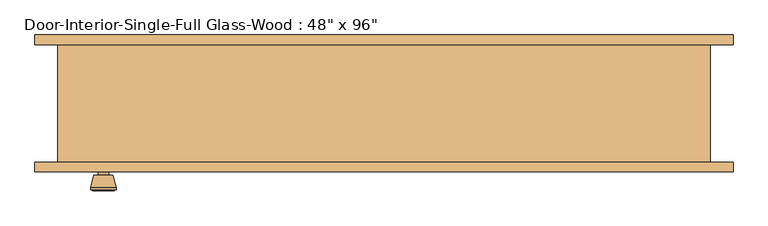
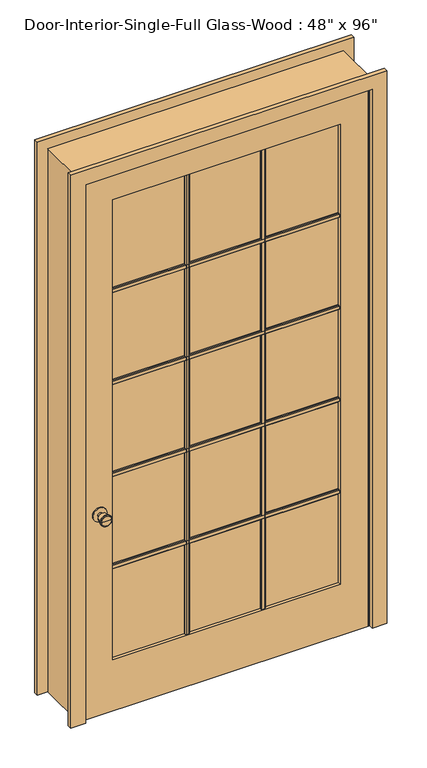
"""IFC4 building model written with IfcOpenShell, lengths in millimetres: door geometry."""

from ifc_helpers import new_model, si_unit, point, frame, frame_2d, origin, place, context, project, spatial, polyline, circle_curve, trimmed, segment, composite_curve, outline, extrude, faceted_brep, source, transform, mapped, element, save
from ifc_brep_helpers import plane_surface, cylinder_surface, revolved_surface, advanced_brep


def door_6ee39103(model_context):
    return source(origin(), model_context, "Body", "SolidModel", [
        extrude(outline(polyline([(-97.155, 1911.35), (-97.155, 1892.3), (-103.505, 1892.3), (-106.68, 1895.475), (-106.68, 1908.175), (-103.505, 1911.35), (-97.155, 1911.35)])), frame((-488.95, 0.0, 0.0), z_axis=(1.0, 0.0, 0.0), x_axis=(0.0, 1.0, 0.0)), (0.0, 0.0, 1.0), 977.9),
        extrude(outline(polyline([(-97.155, 1493.8375), (-97.155, 1474.7875), (-103.505, 1474.7875), (-106.68, 1477.9625), (-106.68, 1490.6625), (-103.505, 1493.8375), (-97.155, 1493.8375)])), frame((-488.95, 0.0, 0.0), z_axis=(1.0, 0.0, 0.0), x_axis=(0.0, 1.0, 0.0)), (0.0, 0.0, 1.0), 977.9),
        extrude(outline(polyline([(-97.155, 1076.325), (-97.155, 1057.275), (-103.505, 1057.275), (-106.68, 1060.45), (-106.68, 1073.15), (-103.505, 1076.325), (-97.155, 1076.325)])), frame((-488.95, 0.0, 0.0), z_axis=(1.0, 0.0, 0.0), x_axis=(0.0, 1.0, 0.0)), (0.0, 0.0, 1.0), 977.9),
        extrude(outline(polyline([(-97.155, 658.8125), (-97.155, 639.7625), (-103.505, 639.7625), (-106.68, 642.9375), (-106.68, 655.6375), (-103.505, 658.8125), (-97.155, 658.8125)])), frame((-488.95, 0.0, 0.0), z_axis=(1.0, 0.0, 0.0), x_axis=(0.0, 1.0, 0.0)), (0.0, 0.0, 1.0), 977.9),
        extrude(outline(polyline([(153.4583333, -97.155), (172.5083333, -97.155), (172.5083333, -103.505), (169.3333333, -106.68), (156.6333333, -106.68), (153.4583333, -103.505), (153.4583333, -97.155)])), frame((0.0, 0.0, 231.775), z_axis=(0.0, 0.0, 1.0), x_axis=(1.0, 0.0, 0.0)), (0.0, 0.0, 1.0), 2087.5625),
        extrude(outline(polyline([(-172.5083333, -97.155), (-153.4583333, -97.155), (-153.4583333, -103.505), (-156.6333333, -106.68), (-169.3333333, -106.68), (-172.5083333, -103.505), (-172.5083333, -97.155)])), frame((0.0, 0.0, 231.775), z_axis=(0.0, 0.0, 1.0), x_axis=(1.0, 0.0, 0.0)), (0.0, 0.0, 1.0), 2087.5625),
        extrude(outline(polyline([(-90.17, 1911.35), (-83.82, 1911.35), (-80.645, 1908.175), (-80.645, 1895.475), (-83.82, 1892.3), (-90.17, 1892.3), (-90.17, 1911.35)])), frame((-488.95, 0.0, 0.0), z_axis=(1.0, 0.0, 0.0), x_axis=(0.0, 1.0, 0.0)), (0.0, 0.0, 1.0), 977.9),
        extrude(outline(polyline([(-90.17, 1493.8375), (-83.82, 1493.8375), (-80.645, 1490.6625), (-80.645, 1477.9625), (-83.82, 1474.7875), (-90.17, 1474.7875), (-90.17, 1493.8375)])), frame((-488.95, 0.0, 0.0), z_axis=(1.0, 0.0, 0.0), x_axis=(0.0, 1.0, 0.0)), (0.0, 0.0, 1.0), 977.9),
        extrude(outline(polyline([(-90.17, 1076.325), (-83.82, 1076.325), (-80.645, 1073.15), (-80.645, 1060.45), (-83.82, 1057.275), (-90.17, 1057.275), (-90.17, 1076.325)])), frame((-488.95, 0.0, 0.0), z_axis=(1.0, 0.0, 0.0), x_axis=(0.0, 1.0, 0.0)), (0.0, 0.0, 1.0), 977.9),
        extrude(outline(polyline([(-90.17, 658.8125), (-83.82, 658.8125), (-80.645, 655.6375), (-80.645, 642.9375), (-83.82, 639.7625), (-90.17, 639.7625), (-90.17, 658.8125)])), frame((-488.95, 0.0, 0.0), z_axis=(1.0, 0.0, 0.0), x_axis=(0.0, 1.0, 0.0)), (0.0, 0.0, 1.0), 977.9),
        extrude(outline(polyline([(153.4583333, -90.17), (153.4583333, -83.82), (156.6333333, -80.645), (169.3333333, -80.645), (172.5083333, -83.82), (172.5083333, -90.17), (153.4583333, -90.17)])), frame((0.0, 0.0, 231.775), z_axis=(0.0, 0.0, 1.0), x_axis=(1.0, 0.0, 0.0)), (0.0, 0.0, 1.0), 2087.5625),
        extrude(outline(polyline([(-172.5083333, -90.17), (-172.5083333, -83.82), (-169.3333333, -80.645), (-156.6333333, -80.645), (-153.4583333, -83.82), (-153.4583333, -90.17), (-172.5083333, -90.17)])), frame((0.0, 0.0, 231.775), z_axis=(0.0, 0.0, 1.0), x_axis=(1.0, 0.0, 0.0)), (0.0, 0.0, 1.0), 2087.5625),
        advanced_brep(
        [(-546.1, -70.2, 914.4), (-556.1, -70.2, 914.4), (-536.1, -70.2, 914.4), (-525.6241324, -21.2, 914.4), (-566.5758676, -21.2, 914.4), (-546.1, -21.2, 914.4), (-521.1, -23.0278681, 914.4), (-571.1, -23.0278681, 914.4), (-521.1, -26.4915463, 914.4), (-571.1, -26.4915463, 914.4), (-527.463764, -51.2, 914.4), (-564.736236, -51.2, 914.4), (-536.1, -51.2, 914.4), (-556.1, -51.2, 914.4)],
        [
            (0, 1),
            (1, 2, circle_curve(frame((-546.1, -70.2, 914.4), z_axis=(0.0, -1.0, 0.0), x_axis=(-1.0, 0.0, 0.0)), 10.0)),
            (2, 0),
            (2, 1, circle_curve(frame((-546.1, -70.2, 914.4), z_axis=(0.0, -1.0, 0.0), x_axis=(-1.0, 0.0, 0.0)), 10.0)),
            (3, 4, circle_curve(frame((-546.1, -21.2, 914.4), z_axis=(0.0, 1.0, 0.0), x_axis=(-1.0, 0.0, 0.0)), 20.4758676)),
            (4, 5),
            (5, 3),
            (4, 3, circle_curve(frame((-546.1, -21.2, 914.4), z_axis=(0.0, 1.0, 0.0), x_axis=(-1.0, 0.0, 0.0)), 20.4758676)),
            (6, 7, circle_curve(frame((-546.1, -23.0278681, 914.4), z_axis=(0.0, 1.0, 0.0), x_axis=(-1.0, 0.0, 0.0)), 25.0)),
            (7, 4),
            (3, 6),
            (7, 6, circle_curve(frame((-546.1, -23.0278681, 914.4), z_axis=(0.0, 1.0, 0.0), x_axis=(-1.0, 0.0, 0.0)), 25.0)),
            (8, 9, circle_curve(frame((-546.1, -26.4915463, 914.4), z_axis=(0.0, 1.0, 0.0), x_axis=(-1.0, 0.0, 0.0)), 25.0)),
            (9, 7),
            (6, 8),
            (9, 8, circle_curve(frame((-546.1, -26.4915463, 914.4), z_axis=(0.0, 1.0, 0.0), x_axis=(-1.0, 0.0, 0.0)), 25.0)),
            (10, 11, circle_curve(frame((-546.1, -51.2, 914.4), z_axis=(0.0, 1.0, 0.0), x_axis=(-1.0, 0.0, 0.0)), 18.636236)),
            (11, 9),
            (8, 10),
            (11, 10, circle_curve(frame((-546.1, -51.2, 914.4), z_axis=(0.0, 1.0, 0.0), x_axis=(-1.0, 0.0, 0.0)), 18.636236)),
            (12, 13, circle_curve(frame((-546.1, -51.2, 914.4), z_axis=(0.0, 1.0, 0.0), x_axis=(-1.0, 0.0, 0.0)), 10.0)),
            (13, 11),
            (10, 12),
            (13, 12, circle_curve(frame((-546.1, -51.2, 914.4), z_axis=(0.0, 1.0, 0.0), x_axis=(-1.0, 0.0, 0.0)), 10.0)),
            (1, 13),
            (12, 2),
        ],
        [
            plane_surface(frame((-546.1, -70.2, 914.4), z_axis=(0.0, -1.0, 0.0), x_axis=(-1.0, 0.0, 0.0))),
            plane_surface(frame((-546.1, -21.2, 914.4), z_axis=(0.0, 1.0, 0.0), x_axis=(-1.0, 0.0, 0.0))),
            revolved_surface(polyline([(-566.5758676, -21.2, 914.4), (-571.1, -23.0278681, 914.4)]), (-546.1, -70.2, 914.4), (0.0, -1.0, 0.0)),
            cylinder_surface(frame((-546.1, -70.2, 914.4), z_axis=(0.0, -1.0, 0.0), x_axis=(-1.0, 0.0, 0.0)), 25.0),
            revolved_surface(polyline([(-571.1, -26.4915463, 914.4), (-564.736236, -51.2, 914.4)]), (-546.1, -70.2, 914.4), (0.0, -1.0, 0.0)),
            plane_surface(frame((-546.1, -51.2, 914.4), z_axis=(0.0, -1.0, 0.0), x_axis=(-1.0, 0.0, 0.0))),
            cylinder_surface(frame((-546.1, -70.2, 914.4), z_axis=(0.0, -1.0, 0.0), x_axis=(-1.0, 0.0, 0.0)), 10.0),
        ],
        [
            (0, [[1, 2, 3]]),
            (0, [[-3, 4, -1]]),
            (1, [[5, 6, 7]]),
            (1, [[8, -7, -6]]),
            (2, [[9, 10, -5, 11]]),
            (2, [[12, -11, -8, -10]]),
            (3, [[13, 14, -9, 15]]),
            (3, [[16, -15, -12, -14]]),
            (4, [[17, 18, -13, 19]]),
            (4, [[20, -19, -16, -18]]),
            (5, [[21, 22, -17, 23]]),
            (5, [[24, -23, -20, -22]]),
            (6, [[-2, 25, -21, 26]]),
            (6, [[-4, -26, -24, -25]]),
        ],
    ),
        extrude(outline(composite_curve([segment(trimmed(circle_curve(frame_2d((914.4, -546.1)), 30.0), [point((914.4, -576.1))], [point((914.4, -516.1))], False, "CARTESIAN"), True, "CONTINUOUS"), segment(trimmed(circle_curve(frame_2d((914.4, -546.1)), 30.0), [point((914.4, -516.1))], [point((914.4, -576.1))], False, "CARTESIAN"), True, "CONTINUOUS")], self_intersect=False)), frame((0.0, -76.2, 0.0), z_axis=(0.0, 1.0, 0.0), x_axis=(0.0, 0.0, 1.0)), (0.0, 0.0, 1.0), 6.0),
        advanced_brep(
        [(-546.1, -117.125, 914.4), (-536.1, -117.125, 914.4), (-556.1, -117.125, 914.4), (-525.6241324, -166.125, 914.4), (-546.1, -166.125, 914.4), (-566.5758676, -166.125, 914.4), (-521.1, -164.2971319, 914.4), (-571.1, -164.2971319, 914.4), (-521.1, -160.8334537, 914.4), (-571.1, -160.8334537, 914.4), (-527.463764, -136.125, 914.4), (-564.736236, -136.125, 914.4), (-536.1, -136.125, 914.4), (-556.1, -136.125, 914.4)],
        [
            (0, 1),
            (1, 2, circle_curve(frame((-546.1, -117.125, 914.4), z_axis=(0.0, 1.0, 0.0), x_axis=(-1.0, 0.0, 0.0)), 10.0)),
            (2, 0),
            (2, 1, circle_curve(frame((-546.1, -117.125, 914.4), z_axis=(0.0, 1.0, 0.0), x_axis=(-1.0, 0.0, 0.0)), 10.0)),
            (3, 4),
            (4, 5),
            (5, 3, circle_curve(frame((-546.1, -166.125, 914.4), z_axis=(0.0, -1.0, 0.0), x_axis=(-1.0, 0.0, 0.0)), 20.4758676)),
            (3, 5, circle_curve(frame((-546.1, -166.125, 914.4), z_axis=(0.0, -1.0, 0.0), x_axis=(-1.0, 0.0, 0.0)), 20.4758676)),
            (6, 3),
            (5, 7),
            (7, 6, circle_curve(frame((-546.1, -164.2971319, 914.4), z_axis=(0.0, -1.0, 0.0), x_axis=(-1.0, 0.0, 0.0)), 25.0)),
            (6, 7, circle_curve(frame((-546.1, -164.2971319, 914.4), z_axis=(0.0, -1.0, 0.0), x_axis=(-1.0, 0.0, 0.0)), 25.0)),
            (8, 6),
            (7, 9),
            (9, 8, circle_curve(frame((-546.1, -160.8334537, 914.4), z_axis=(0.0, -1.0, 0.0), x_axis=(-1.0, 0.0, 0.0)), 25.0)),
            (8, 9, circle_curve(frame((-546.1, -160.8334537, 914.4), z_axis=(0.0, -1.0, 0.0), x_axis=(-1.0, 0.0, 0.0)), 25.0)),
            (10, 8),
            (9, 11),
            (11, 10, circle_curve(frame((-546.1, -136.125, 914.4), z_axis=(0.0, -1.0, 0.0), x_axis=(-1.0, 0.0, 0.0)), 18.636236)),
            (10, 11, circle_curve(frame((-546.1, -136.125, 914.4), z_axis=(0.0, -1.0, 0.0), x_axis=(-1.0, 0.0, 0.0)), 18.636236)),
            (12, 10),
            (11, 13),
            (13, 12, circle_curve(frame((-546.1, -136.125, 914.4), z_axis=(0.0, -1.0, 0.0), x_axis=(-1.0, 0.0, 0.0)), 10.0)),
            (12, 13, circle_curve(frame((-546.1, -136.125, 914.4), z_axis=(0.0, -1.0, 0.0), x_axis=(-1.0, 0.0, 0.0)), 10.0)),
            (1, 12),
            (13, 2),
        ],
        [
            plane_surface(frame((-546.1, -117.125, 914.4), z_axis=(0.0, 1.0, 0.0), x_axis=(-1.0, 0.0, 0.0))),
            plane_surface(frame((-546.1, -166.125, 914.4), z_axis=(0.0, -1.0, 0.0), x_axis=(-1.0, 0.0, 0.0))),
            revolved_surface(polyline([(-566.5758676, -166.125, 914.4), (-571.1, -164.2971319, 914.4)]), (-546.1, -117.125, 914.4), (0.0, 1.0, 0.0)),
            cylinder_surface(frame((-546.1, -117.125, 914.4), z_axis=(0.0, 1.0, 0.0), x_axis=(-1.0, 0.0, 0.0)), 25.0),
            revolved_surface(polyline([(-571.1, -160.8334537, 914.4), (-564.736236, -136.125, 914.4)]), (-546.1, -117.125, 914.4), (0.0, 1.0, 0.0)),
            plane_surface(frame((-546.1, -136.125, 914.4), z_axis=(0.0, 1.0, 0.0), x_axis=(-1.0, 0.0, 0.0))),
            cylinder_surface(frame((-546.1, -117.125, 914.4), z_axis=(0.0, 1.0, 0.0), x_axis=(-1.0, 0.0, 0.0)), 10.0),
        ],
        [
            (0, [[1, 2, 3]]),
            (0, [[-3, 4, -1]]),
            (1, [[5, 6, 7]]),
            (1, [[-6, -5, 8]]),
            (2, [[9, -7, 10, 11]]),
            (2, [[-10, -8, -9, 12]]),
            (3, [[13, -11, 14, 15]]),
            (3, [[-14, -12, -13, 16]]),
            (4, [[17, -15, 18, 19]]),
            (4, [[-18, -16, -17, 20]]),
            (5, [[21, -19, 22, 23]]),
            (5, [[-22, -20, -21, 24]]),
            (6, [[25, -23, 26, -2]]),
            (6, [[-26, -24, -25, -4]]),
        ],
    ),
        extrude(outline(composite_curve([segment(trimmed(circle_curve(frame_2d((914.4, -546.1)), 30.0), [point((914.4, -576.1))], [point((914.4, -516.1))], False, "CARTESIAN"), True, "CONTINUOUS"), segment(trimmed(circle_curve(frame_2d((914.4, -546.1)), 30.0), [point((914.4, -516.1))], [point((914.4, -576.1))], False, "CARTESIAN"), True, "CONTINUOUS")], self_intersect=False)), frame((0.0, -117.125, 0.0), z_axis=(0.0, 1.0, 0.0), x_axis=(0.0, 0.0, 1.0)), (0.0, 0.0, 1.0), 6.0),
        faceted_brep([(635.0, -111.125, 0.0), (609.6, -111.125, 0.0), (609.6, -76.2, 0.0), (596.9, -76.2, 0.0), (596.9, -41.275, 0.0), (609.6, -41.275, 0.0), (609.6, 117.475, 0.0), (635.0, 117.475, 0.0), (635.0, 117.475, 2463.8), (635.0, -111.125, 2463.8), (609.6, 117.475, 2438.4), (-609.6, 117.475, 2438.4), (-609.6, 117.475, 0.0), (-635.0, 117.475, 0.0), (-635.0, 117.475, 2463.8), (609.6, -41.275, 2438.4), (596.9, -41.275, 2425.7), (-596.9, -41.275, 2425.7), (-596.9, -41.275, 0.0), (-609.6, -41.275, 0.0), (-609.6, -41.275, 2438.4), (596.9, -76.2, 2425.7), (609.6, -76.2, 2438.4), (-609.6, -76.2, 2438.4), (-609.6, -76.2, 0.0), (-596.9, -76.2, 0.0), (-596.9, -76.2, 2425.7), (609.6, -111.125, 2438.4), (-635.0, -111.125, 2463.8), (-635.0, -111.125, 0.0), (-609.6, -111.125, 0.0), (-609.6, -111.125, 2438.4)], [[[0, 1, 2, 3, 4, 5, 6, 7]], [[7, 8, 9, 0]], [[6, 10, 11, 12, 13, 14, 8, 7]], [[5, 15, 10, 6]], [[4, 16, 17, 18, 19, 20, 15, 5]], [[3, 21, 16, 4]], [[2, 22, 23, 24, 25, 26, 21, 3]], [[1, 27, 22, 2]], [[0, 9, 28, 29, 30, 31, 27, 1]], [[8, 14, 28, 9]], [[15, 20, 11, 10]], [[21, 26, 17, 16]], [[27, 31, 23, 22]], [[29, 13, 12, 19, 18, 25, 24, 30]], [[14, 13, 29, 28]], [[20, 19, 12, 11]], [[26, 25, 18, 17]], [[31, 30, 24, 23]]]),
        extrude(outline(polyline([(2438.4, -609.6), (0.0, -609.6), (0.0, 609.6), (2438.4, 609.6), (2438.4, -609.6)]), holes=[polyline([(2319.3375, -488.95), (2319.3375, 488.95), (231.775, 488.95), (231.775, -488.95), (2319.3375, -488.95)])]), frame((0.0, -111.125, 0.0), z_axis=(0.0, 1.0, 0.0), x_axis=(0.0, 0.0, 1.0)), (0.0, 0.0, 1.0), 34.925),
        extrude(outline(polyline([(488.95, -90.17), (488.95, -97.155), (-488.95, -97.155), (-488.95, -90.17), (488.95, -90.17)])), frame((0.0, 0.0, 231.775), z_axis=(0.0, 0.0, 1.0), x_axis=(1.0, 0.0, 0.0)), (0.0, 0.0, 1.0), 2087.5625),
        extrude(outline(polyline([(0.0, 679.45), (2508.25, 679.45), (2508.25, -679.45), (0.0, -679.45), (0.0, -615.95), (2444.75, -615.95), (2444.75, 615.95), (0.0, 615.95), (0.0, 679.45)])), frame((0.0, -130.175, 0.0), z_axis=(0.0, 1.0, 0.0), x_axis=(0.0, 0.0, 1.0)), (0.0, 0.0, 1.0), 19.05),
        extrude(outline(polyline([(0.0, 679.45), (2508.25, 679.45), (2508.25, -679.45), (0.0, -679.45), (0.0, -615.95), (2444.75, -615.95), (2444.75, 615.95), (0.0, 615.95), (0.0, 679.45)])), frame((0.0, 117.475, 0.0), z_axis=(0.0, 1.0, 0.0), x_axis=(0.0, 0.0, 1.0)), (0.0, 0.0, 1.0), 19.05),
    ])


if __name__ == "__main__":
    model = new_model("IFC4")
    model_context = context("Model", 3, world=origin())
    ifc_project = project(units=[si_unit("LENGTHUNIT", "METRE", prefix="MILLI")], contexts=[model_context])
    site = spatial("IfcSite", under=ifc_project)
    building = spatial("IfcBuilding", under=site)
    placement = place(None, origin())
    door_shape = door_6ee39103(model_context)
    element("IfcDoor", 1, ObjectType="Door-Interior-Single-Full Glass-Wood : 48\" x 96\"", at=placement, inside=building, context=model_context, shape_type="MappedRepresentation", body=[
        mapped(door_shape, transform((0.0, 0.0, 0.0), x_axis=(1.0, 0.0, 0.0), y_axis=(0.0, 1.0, 0.0), z_axis=(0.0, 0.0, 1.0))),
    ])
    save(model, "model.ifc")

# Revit data of these elements
# Type "Door-Interior-Single-Full Glass-Wood : 48\" x 96\""
#   Type Mark = "8"
#   Assembly Code = "C1020300"
#   Analytic Construction = "Wood frame with single clear glass"
#   Top Rail = 0' - 4 11/16"
#   Thickness = 0' - 1 3/8"
#   Thermal Resistance (R) = 1.0102 (h·ft²·°F)/BTU
#   Swing Angle [instance default] = 90.00°
#   Stiles = 0' - 4 3/4"
#   Rough Width = 4' - 2"
#   Rough Height = 8' - 1"
#   Height = 8' - 0"
#   Width = 4' - 0"
#   Heat Transfer Coefficient (U) = 0.9900 BTU/(h·ft²·°F)
#   Bottom Rail = 0' - 9 1/8"
#   Show Grill [instance default] = yes
#   Trim Material = Cherry
#   Panel Material = Cherry
#   Frame Material = Cherry
#   Door Handle Material = Aluminum
#   Visual Light Transmittance = 0
#   Solar Heat Gain Coefficient = 0
#   Wall Closure = (empty or 0)
#   Function = (empty or 0)
# Element 1 (IfcDoor, "Door-Interior-Single-Full Glass-Wood : 48\" x 96\"")
#   Materials on its faces: "Cherry", "Aluminum", "Glass"
# Materials
#   "Cherry": class "Wood", colour RGB 226 177 128, transparency 0, Description = "Prunus Serotina", Cost = 0
#   "Aluminum": class "Metal", colour RGB 247 247 247, transparency 0, Description = "Aluminum 6061", Cost = 0
#   "Glass": class "Glass", colour RGB 0 128 192, transparency 0.75, Description = "Soda Lime Glass", Cost = 0
